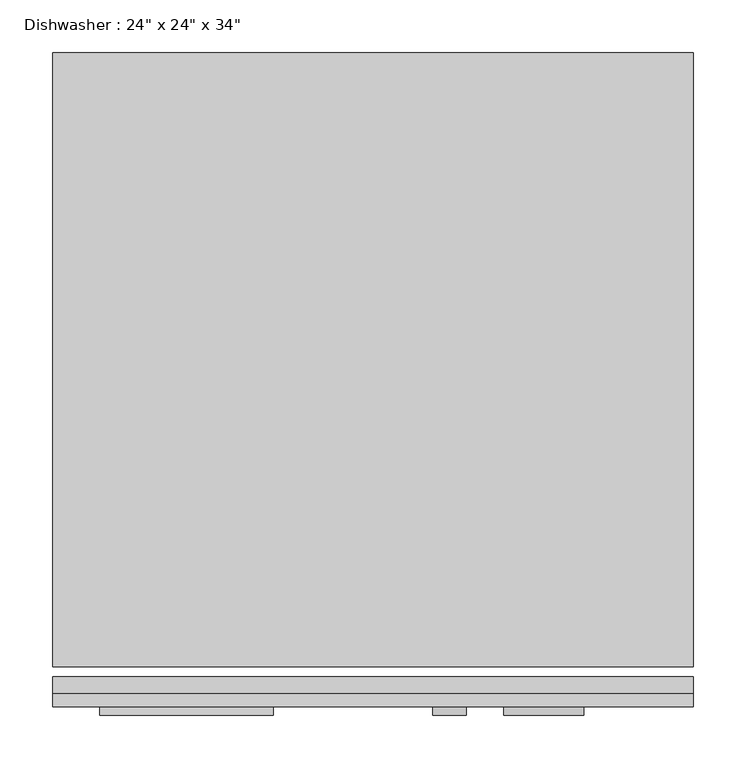
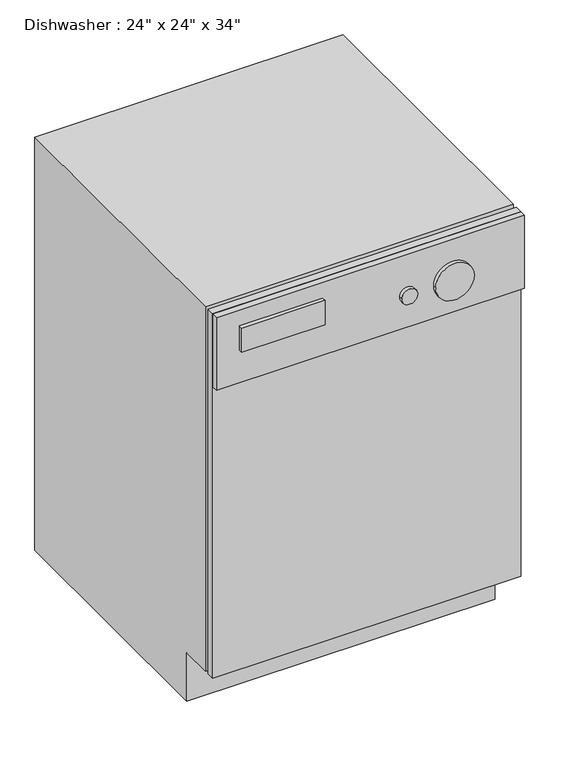
"""IFC4 building model written with IfcOpenShell, lengths in millimetres: proxy geometry."""

from ifc_helpers import new_model, si_unit, point, frame, frame_2d, origin, place, context, project, spatial, polyline, circle_curve, trimmed, segment, composite_curve, outline, extrude, source, transform, mapped, element, save


def proxy_45b28599(model_context):
    return source(origin(), model_context, "Body", "SweptSolid", [
        extrude(outline(polyline([(687.1174685, -38.3504352), (77.5174685, -38.3504352), (77.5174685, -22.4754352), (687.1174685, -22.4754352), (687.1174685, -38.3504352)])), frame((0.0, 0.0, 101.6), z_axis=(0.0, 0.0, 1.0), x_axis=(1.0, 0.0, 0.0)), (0.0, 0.0, 1.0), 762.0),
        extrude(outline(polyline([(687.1174685, -38.3504352), (687.1174685, -51.0504352), (77.5174685, -51.0504352), (77.5174685, -38.3504352), (687.1174685, -38.3504352)])), frame((0.0, 0.0, 711.2), z_axis=(0.0, 0.0, 1.0), x_axis=(1.0, 0.0, 0.0)), (0.0, 0.0, 1.0), 152.4),
        extrude(outline(polyline([(571.2495648, 0.0), (50.5495648, 0.0), (50.5495648, 101.6), (-12.9504352, 101.6), (-12.9504352, 863.6), (571.2495648, 863.6), (571.2495648, 0.0)])), frame((77.5174685, 0.0, 0.0), z_axis=(1.0, 0.0, 0.0), x_axis=(0.0, 1.0, 0.0)), (0.0, 0.0, 1.0), 609.6),
        extrude(outline(polyline([(287.6378068, -59.1863727), (122.5378068, -59.1863727), (122.5378068, -51.0504352), (287.6378068, -51.0504352), (287.6378068, -59.1863727)])), frame((0.0, 0.0, 780.0846419), z_axis=(0.0, 0.0, 1.0), x_axis=(1.0, 0.0, 0.0)), (0.0, 0.0, 1.0), 50.8),
        extrude(outline(composite_curve([segment(trimmed(circle_curve(frame_2d((780.0846419, 544.7247133)), 38.1), [point((780.0846419, 506.6247133))], [point((780.0846419, 582.8247133))], False, "CARTESIAN"), True, "CONTINUOUS"), segment(trimmed(circle_curve(frame_2d((780.0846419, 544.7247133)), 38.1), [point((780.0846419, 582.8247133))], [point((780.0846419, 506.6247133))], False, "CARTESIAN"), True, "CONTINUOUS")], self_intersect=False)), frame((0.0, -59.1863727, 0.0), z_axis=(0.0, 1.0, 0.0), x_axis=(0.0, 0.0, 1.0)), (0.0, 0.0, 1.0), 8.1359375),
        extrude(outline(composite_curve([segment(trimmed(circle_curve(frame_2d((780.0846419, 455.195318)), 15.875), [point((780.0846419, 439.320318))], [point((780.0846419, 471.070318))], False, "CARTESIAN"), True, "CONTINUOUS"), segment(trimmed(circle_curve(frame_2d((780.0846419, 455.195318)), 15.875), [point((780.0846419, 471.070318))], [point((780.0846419, 439.320318))], False, "CARTESIAN"), True, "CONTINUOUS")], self_intersect=False)), frame((0.0, -59.1863727, 0.0), z_axis=(0.0, 1.0, 0.0), x_axis=(0.0, 0.0, 1.0)), (0.0, 0.0, 1.0), 8.1359375),
    ])


if __name__ == "__main__":
    model = new_model("IFC4")
    model_context = context("Model", 3, world=origin())
    ifc_project = project(units=[si_unit("LENGTHUNIT", "METRE", prefix="MILLI")], contexts=[model_context])
    site = spatial("IfcSite", under=ifc_project)
    building = spatial("IfcBuilding", under=site)
    placement = place(None, origin())
    proxy_shape = proxy_45b28599(model_context)
    element("IfcBuildingElementProxy", 1, Name="Dishwasher : 24\" x 24\" x 34\"", ObjectType="Dishwasher : 24\" x 24\" x 34\"", at=placement, inside=building, context=model_context, shape_type="MappedRepresentation", body=[
        mapped(proxy_shape, transform((0.0, 0.0, 0.0), x_axis=(1.0, 0.0, 0.0), y_axis=(0.0, 1.0, 0.0), z_axis=(0.0, 0.0, 1.0))),
    ])
    save(model, "model.ifc")

# Revit data of these elements
# Type "Dishwasher : 24\" x 24\" x 34\""
#   Label = "DW"
#   Assembly Code = "E1090400"
#   Depth = 2' - 0"
#   Height = 2' - 10"
#   Width = 2' - 0"
#   Dishwasher Material = Steel, Paint Finish, Ivory, Glossy
#   Panel Face Material = Plastic, Opaque Black
#   Default Elevation = 0
# Element 1 (IfcBuildingElementProxy, "Dishwasher : 24\" x 24\" x 34\"")
#   Materials on its faces: "Steel, Paint Finish, Ivory, Glossy", "Plastic, Opaque Black"
# Materials
#   "Steel, Paint Finish, Ivory, Glossy": class "Metal", colour RGB 247 247 239, transparency 0, Description = "Steel, paint finish, ivory, glossy", Cost = 0
#   "Plastic, Opaque Black": class "Plastic", colour RGB 0 0 0, transparency 0.7, Description = "Plastic, generic, opaque black", Cost = 0
